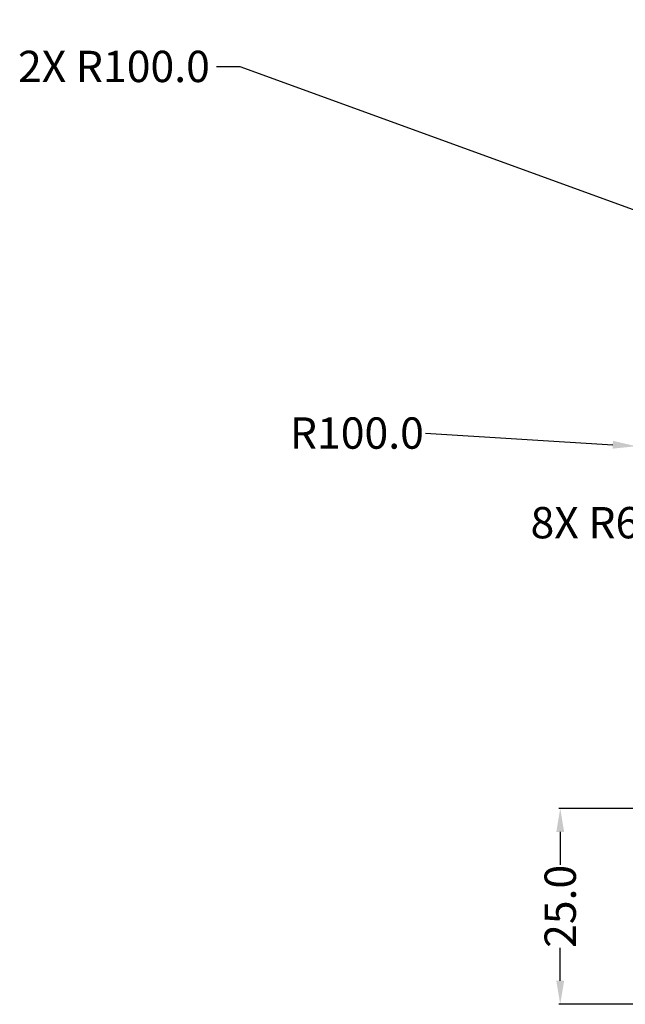
# Model space of a CAD drawing. Units: millimetres. Extents: x 285 to 514, y 588 to 771.
# Tile 1 of 3: x 285 to 363, y 626 to 752. Entities that reach past the tile are written whole.
import ezdxf

# ---------------------------------------------------------------- set-up
doc = ezdxf.new("R2010")
doc.units = ezdxf.units.MM
doc.header["$MEASUREMENT"] = 0
doc.layers.add('M-DIMS', color=2, linetype='Continuous', lineweight=25)
doc.styles.get("Standard").update_dxf_attribs({"font": 'arial.ttf'})
doc.dimstyles.get("Standard").update_dxf_attribs({"dimtxt": 4, "dimasz": 3, "dimexe": 0.18, "dimexo": 0.0625, "dimgap": 0.09, "dimtad": 0, "dimtoh": 1, "dimdec": 1, "dimzin": 0, "dimdsep": 46, "dimtxsty": 'Standard', "dimcen": 0.09, "dimadec": 0, "dimazin": 0, "dimtfac": 1, "dimtdec": 1, "dimtofl": 0, "dimtmove": 0, "dimatfit": 3, "dimfxl": 1, "dimtolj": 1, "dimtzin": 0, "dimarcsym": 0})

# ---------------------------------------------------------------- blocks, each defined once
blk = doc.blocks.new('*D3')
at = {"layer": 'Defpoints', "color": 0, "transparency": 16777216}
for p in [(364.13, 697.39), (463.94, 691.15)]:
    blk.add_point(p, dxfattribs=at)
at = {"layer": 'M-DIMS', "color": 0, "lineweight": -2, "transparency": 16777216}
for p, q in [((337.25, 699.07), (361.14, 697.58)), ((463.85, 691.15), (464.03, 691.15)), ((463.94, 691.06), (463.94, 691.24))]:
    blk.add_line(p, q, dxfattribs=at)
at = {"layer": 'M-DIMS', "color": 0, "transparency": 16777216}
blk.add_solid([(361.17, 698.07), (361.11, 697.08), (364.13, 697.39)], dxfattribs=at)
at = {"layer": 'M-DIMS', "color": 0, "transparency": 16777216, "insert": (328.5, 699.07), "char_height": 4, "attachment_point": 5}
blk.add_mtext('\\A1;R100.0', dxfattribs=at)
blk = doc.blocks.new('*D23')
at = {"layer": 'Defpoints', "color": 0, "transparency": 16777216}
for p in [(407.29, 651.15), (354.44, 626.15), (407.29, 626.15)]:
    blk.add_point(p, dxfattribs=at)
at = {"layer": 'M-DIMS', "color": 0, "lineweight": -2, "transparency": 16777216}
for p, q in [((407.22, 651.15), (354.26, 651.15)), ((354.44, 648.15), (354.44, 643.96)), ((354.44, 629.15), (354.44, 633.34)), ((407.22, 626.15), (354.26, 626.15))]:
    blk.add_line(p, q, dxfattribs=at)
at = {"layer": 'M-DIMS', "color": 0, "transparency": 16777216}
for points in [[(353.94, 648.15), (354.94, 648.15), (354.44, 651.15)], [(353.94, 629.15), (354.94, 629.15), (354.44, 626.15)]]:
    blk.add_solid(points, dxfattribs=at)
at = {"layer": 'M-DIMS', "color": 0, "transparency": 16777216, "insert": (354.44, 638.65), "char_height": 4, "attachment_point": 5, "rotation": 90}
blk.add_mtext('\\A1;25.0', dxfattribs=at)
blk = doc.blocks.new('*D30')
at = {"layer": 'Defpoints', "color": 0, "transparency": 16777216}
for p in [(377.04, 683.39), (381.29, 679.15)]:
    blk.add_point(p, dxfattribs=at)
at = {"layer": 'M-DIMS', "color": 0, "lineweight": -2, "transparency": 16777216}
for p, q in [((369.8, 687.63), (372.8, 687.63)), ((372.8, 687.63), (374.92, 685.51)), ((381.2, 679.15), (381.38, 679.15)), ((381.29, 679.06), (381.29, 679.24))]:
    blk.add_line(p, q, dxfattribs=at)
at = {"layer": 'M-DIMS', "color": 0, "transparency": 16777216}
blk.add_solid([(375.28, 685.87), (374.57, 685.16), (377.04, 683.39)], dxfattribs=at)
at = {"layer": 'M-DIMS', "color": 0, "transparency": 16777216, "insert": (359.86, 687.63), "char_height": 4, "attachment_point": 5}
blk.add_mtext('\\A1;8X R6.0', dxfattribs=at)
blk = doc.blocks.new('*D33')
at = {"layer": 'Defpoints', "color": 0, "transparency": 16777216}
for p in [(369.97, 725.35), (463.94, 691.15)]:
    blk.add_point(p, dxfattribs=at)
at = {"layer": 'M-DIMS', "color": 0, "lineweight": -2, "transparency": 16777216}
for p, q in [((310.59, 745.87), (313.59, 745.87)), ((313.59, 745.87), (367.15, 726.38)), ((463.85, 691.15), (464.03, 691.15)), ((463.94, 691.06), (463.94, 691.24))]:
    blk.add_line(p, q, dxfattribs=at)
at = {"layer": 'M-DIMS', "color": 0, "transparency": 16777216}
blk.add_solid([(367.32, 726.85), (366.98, 725.91), (369.97, 725.35)], dxfattribs=at)
at = {"layer": 'M-DIMS', "color": 0, "transparency": 16777216, "insert": (297.51, 745.87), "char_height": 4, "attachment_point": 5}
blk.add_mtext('\\A1;2X R100.0', dxfattribs=at)

msp = doc.modelspace()

# ---------------------------------------------------------------- dimensions: what is measured, and where the dimension line sits
at = {"layer": 'M-DIMS'}
dim = msp.add_radius_dim(center=(463.9384, 691.1492), mpoint=(369.9689, 725.3504), text='2X <>', dimstyle='Standard', override={"dimdec": 1, "dimlfac": 1, "dimrnd": 0, "dimzin": 0, "dimdsep": 46, "dimlunit": 2}, dxfattribs=at)
dim.commit()
dim.dimension.update_dxf_attribs({"geometry": '*D33', "text_midpoint": (297.5094, 745.8711), "dimtype": 164})
dim = msp.add_radius_dim(center=(463.9384, 691.1492), mpoint=(364.1332, 697.3881), dimstyle='Standard', override={"dimclrd": 0, "dimclre": 0, "dimclrt": 0}, dxfattribs=at)
dim.commit()
dim.dimension.update_dxf_attribs({"geometry": '*D3', "text_midpoint": (337.251, 699.0685), "dimtype": 164})
dim = msp.add_radius_dim(center=(381.2869, 679.1492), mpoint=(377.0442, 683.3918), text='8X <>', dimstyle='Standard', override={"dimdec": 1, "dimlfac": 1, "dimrnd": 0, "dimzin": 0, "dimdsep": 46, "dimlunit": 2}, dxfattribs=at)
dim.commit()
dim.dimension.update_dxf_attribs({"geometry": '*D30', "text_midpoint": (359.8629, 687.6344)})
dim = msp.add_linear_dim(base=(354.4384, 626.1492), p1=(407.2869, 651.1492), p2=(407.2869, 626.1492), angle=90, dimstyle='Standard', override={"dimdec": 1, "dimlfac": 1, "dimrnd": 0, "dimzin": 0, "dimdsep": 46, "dimlunit": 2}, dxfattribs=at)
dim.commit()
dim.dimension.update_dxf_attribs({"geometry": '*D23', "text_midpoint": (354.4384, 638.6492)})

doc.saveas('drawing.dxf')
